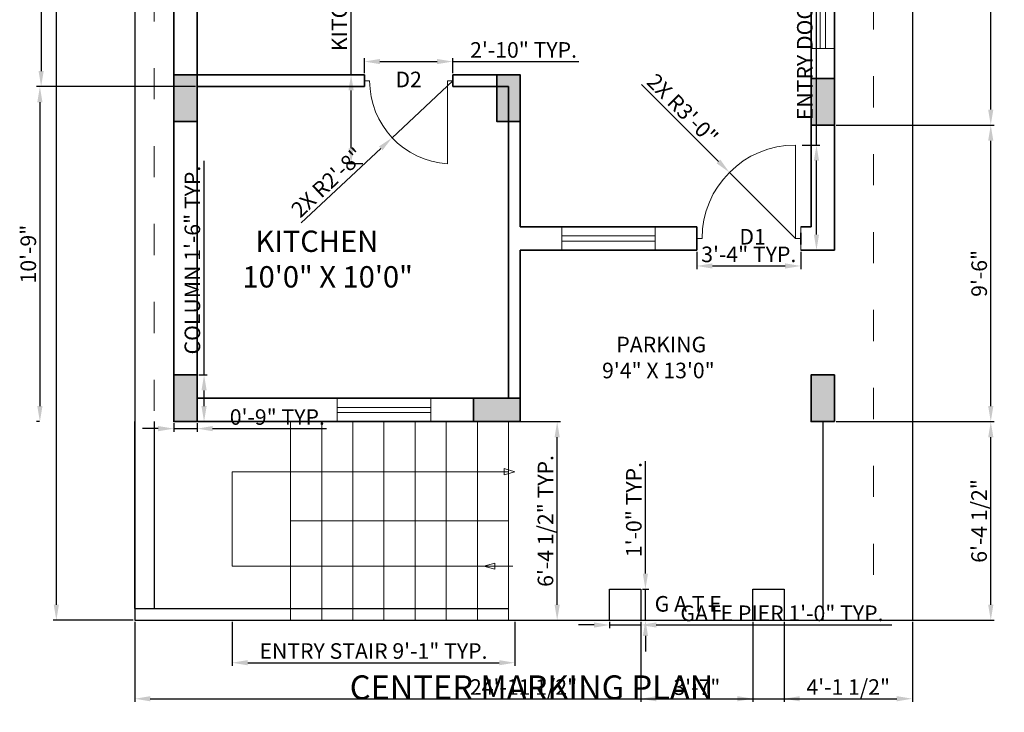
# Model space of a CAD drawing. Units: inches. Extents: x 40559 to 41508, y 131086 to 132358.
# Tile 3 of 5: x 41129 to 41508, y 131086 to 131353. Entities that reach past the tile are written whole.
import ezdxf

# ---------------------------------------------------------------- set-up
doc = ezdxf.new("R2010")
doc.units = ezdxf.units.IN
doc.linetypes.add('ACAD_ISO03W100', pattern=[30, 12, -18])
for name, color, linetype, lineweight in [('A-ANNO-DIMS', 2, 'Continuous', 18), ('A-ANNO-TEXT', 7, 'Continuous', 18), ('A-ANNO-TITL', 7, 'Continuous', 25), ('A-AREA-IDEN', 7, 'Continuous', 18), ('A-FLOR-OVHD', 240, 'ACAD_ISO03W100', 13), ('A-FLOR-STRS', 240, 'Continuous', 18), ('A-SITE-WALL', 7, 'Continuous', 30), ('A-WALL', 7, 'Continuous', 35), ('C-PROP', 7, 'Continuous', 25), ('Doors', 50, 'Continuous', 18), ('Windows', 70, 'Continuous', 18)]:
    doc.layers.add(name, color=color, linetype=linetype, lineweight=lineweight)
doc.layers.add('A-COLS', color=177, linetype='Continuous', lineweight=35, true_color=0x293189)
doc.styles.get("Standard").update_dxf_attribs({"font": 'arial.ttf'})
doc.dimstyles.new('ISO-25', dxfattribs={"dimtxt": 6, "dimasz": 6, "dimexe": 1.25, "dimexo": 0.625, "dimtad": 1, "dimdec": 0, "dimlunit": 3, "dimtxsty": 'Standard', "dimcen": 2.5, "dimclrd": 1, "dimclre": 1, "dimclrt": 2, "dimadec": 0, "dimazin": 0, "dimtfac": 1, "dimtdec": 0, "dimtmove": 0, "dimatfit": 3, "dimfxl": 1, "dimarcsym": 0})

# ---------------------------------------------------------------- blocks, each defined once
blk = doc.blocks.new('*D3')
at = {"layer": 'A-ANNO-DIMS', "color": 0, "lineweight": -2, "transparency": 16777216}
for p, q in [((41187.89, 131457.85), (41136.22, 131457.85)), ((41137.47, 131451.85), (41137.47, 131333.35)), ((41196.89, 131327.35), (41136.22, 131327.35))]:
    blk.add_line(p, q, dxfattribs=at)
at = {"layer": 'A-ANNO-DIMS', "color": 0, "transparency": 16777216}
for points in [[(41136.47, 131451.85), (41138.47, 131451.85), (41137.47, 131457.85)], [(41136.47, 131333.35), (41138.47, 131333.35), (41137.47, 131327.35)]]:
    blk.add_solid(points, dxfattribs=at)
at = {"layer": 'Defpoints', "color": 0, "transparency": 16777216}
for p in [(41188.52, 131457.85), (41137.47, 131327.35), (41197.52, 131327.35)]:
    blk.add_point(p, dxfattribs=at)
at = {"layer": 'A-ANNO-DIMS', "color": 0, "transparency": 16777216, "insert": (41133.78, 131392.6), "char_height": 6, "attachment_point": 5, "rotation": 90}
blk.add_mtext('10\'-11"', dxfattribs=at)
blk = doc.blocks.new('*D4')
at = {"layer": 'A-ANNO-DIMS', "color": 0, "lineweight": -2, "transparency": 16777216}
for p, q in [((41136.84, 131327.35), (41135.73, 131327.35)), ((41136.98, 131321.35), (41136.98, 131204.35)), ((41136.84, 131198.35), (41135.73, 131198.35))]:
    blk.add_line(p, q, dxfattribs=at)
at = {"layer": 'A-ANNO-DIMS', "color": 0, "transparency": 16777216}
for points in [[(41135.98, 131321.35), (41137.98, 131321.35), (41136.98, 131327.35)], [(41135.98, 131204.35), (41137.98, 131204.35), (41136.98, 131198.35)]]:
    blk.add_solid(points, dxfattribs=at)
at = {"layer": 'Defpoints', "color": 0, "transparency": 16777216}
for p in [(41137.47, 131327.35), (41136.98, 131198.35), (41137.47, 131198.35)]:
    blk.add_point(p, dxfattribs=at)
at = {"layer": 'A-ANNO-DIMS', "color": 0, "transparency": 16777216, "insert": (41133.29, 131262.85), "char_height": 6, "attachment_point": 5, "rotation": 90}
blk.add_mtext('10\'-9"', dxfattribs=at)
blk = doc.blocks.new('WIN-36IN')
for p, q in [((0, 5.5), (36, 5.5)), ((0, 3.5), (36, 3.5))]:
    blk.add_line(p, q)
blk.add_lwpolyline([(0, 9), (36, 9), (36, 0), (0, 0)], close=True)
blk = doc.blocks.new('WIN-38IN')
for p, q in [((0, 5.5), (38, 5.5)), ((0, 3.5), (38, 3.5))]:
    blk.add_line(p, q)
blk.add_lwpolyline([(0, 9), (38, 9), (38, 0), (0, 0)], close=True)
blk = doc.blocks.new('DOOR-KITCHEN-34IN')
for p, q in [((34, 29.75), (34, 34.25)), ((34, 29.75), (34, 34.25)), ((0, 32), (2, 32)), ((34, 32), (32, 32)), ((32, 32), (32, 0))]:
    blk.add_line(p, q)
blk.add_arc((34.07, 32), 32.07, 180, 266.3048)
blk = doc.blocks.new('DOOR-ENTRY-40IN')
for p, q in [((38, 4.5), (38, 40.5)), ((40, 9), (40, 0)), ((2, 4.5), (0, 4.5)), ((40, 4.5), (38, 4.5)), ((40, 6.75), (40, 2.25))]:
    blk.add_line(p, q)
blk.add_arc((38, 4.5), 36, 90, 180)
blk = doc.blocks.new('COL-9X18IN')
h = blk.add_hatch(color=256)
h.dxf.hatch_style = 1
h.paths.add_polyline_path([(9, 18), (0, 18), (0, 0), (9, 0)])
blk.add_lwpolyline([(0, 18), (9, 18), (9, 0), (0, 0)], close=True)
blk = doc.blocks.new('ENTRY-STAIR-PLAN')
for p, q in [((22.49, 76.5), (22.49, 0)), ((34.49, 76.5), (34.49, 0)), ((46.49, 76.5), (46.49, 0)), ((58.49, 76.5), (58.49, 0)), ((70.49, 76.5), (70.49, 0)), ((82.49, 76.5), (82.49, 0)), ((94.49, 76.5), (94.49, 0)), ((106.49, 76.5), (106.49, 0)), ((106.49, 57.22), (0, 57.22)), ((0, 57.22), (0, 20.84)), ((97.68, 57.22), (104.71, 57.22)), ((104.71, 57.22), (104.71, 58.4)), ((104.71, 58.4), (108.86, 57.22)), ((104.71, 57.22), (104.71, 56.03)), ((104.71, 56.03), (108.86, 57.22)), ((106.49, 38.25), (22.49, 38.25)), ((0, 20.84), (106.49, 20.84)), ((101.13, 22.03), (96.98, 20.84)), ((101.13, 19.65), (96.98, 20.84)), ((101.13, 20.84), (101.13, 22.03)), ((108.16, 20.84), (101.13, 20.84)), ((101.13, 20.84), (101.13, 19.65))]:
    blk.add_line(p, q)
blk = doc.blocks.new('GATE-PIER-12IN')
for p, q in [((0, 0), (0, 12)), ((0, 12), (12, 12)), ((0, 0), (0, 12)), ((0, 12), (12, 12)), ((12, 12), (12, 0)), ((12, 12), (12, 0))]:
    blk.add_line(p, q)
blk = doc.blocks.new('*D32')
at = {"layer": 'A-ANNO-DIMS', "color": 1, "lineweight": -2, "transparency": 16777216}
for p, q in [((41200.22, 131216.35), (41200.22, 131298.76)), ((41198.14, 131216.35), (41201.47, 131216.35)), ((41200.22, 131204.35), (41200.22, 131210.35)), ((41198.14, 131198.35), (41201.47, 131198.35))]:
    blk.add_line(p, q, dxfattribs=at)
at = {"layer": 'A-ANNO-DIMS', "color": 1, "transparency": 16777216}
for points in [[(41199.22, 131210.35), (41201.22, 131210.35), (41200.22, 131216.35)], [(41199.22, 131204.35), (41201.22, 131204.35), (41200.22, 131198.35)]]:
    blk.add_solid(points, dxfattribs=at)
at = {"layer": 'Defpoints', "color": 0, "transparency": 16777216}
for p in [(41197.52, 131216.35), (41200.22, 131216.35), (41197.52, 131198.35)]:
    blk.add_point(p, dxfattribs=at)
at = {"layer": 'A-ANNO-DIMS', "color": 2, "transparency": 16777216, "insert": (41196.49, 131260.55), "char_height": 6, "attachment_point": 5, "rotation": 90}
blk.add_mtext('COLUMN 1\'-6" TYP.', dxfattribs=at)
blk = doc.blocks.new('*D33')
at = {"layer": 'A-ANNO-DIMS', "color": 1, "lineweight": -2, "transparency": 16777216}
for p, q in [((41182.52, 131195.65), (41176.52, 131195.65)), ((41188.52, 131197.73), (41188.52, 131194.4)), ((41188.52, 131195.65), (41197.52, 131195.65)), ((41197.52, 131197.73), (41197.52, 131194.4)), ((41203.52, 131195.65), (41247.34, 131195.65))]:
    blk.add_line(p, q, dxfattribs=at)
at = {"layer": 'A-ANNO-DIMS', "color": 1, "transparency": 16777216}
for points in [[(41182.52, 131196.65), (41182.52, 131194.65), (41188.52, 131195.65)], [(41203.52, 131196.65), (41203.52, 131194.65), (41197.52, 131195.65)]]:
    blk.add_solid(points, dxfattribs=at)
at = {"layer": 'Defpoints', "color": 0, "transparency": 16777216}
for p in [(41188.52, 131198.35), (41197.52, 131198.35), (41197.52, 131195.65)]:
    blk.add_point(p, dxfattribs=at)
at = {"layer": 'A-ANNO-DIMS', "color": 2, "transparency": 16777216, "insert": (41228.43, 131199.34), "char_height": 6, "attachment_point": 5}
blk.add_mtext('0\'-9" TYP.', dxfattribs=at)
blk = doc.blocks.new('*D42')
at = {"layer": 'A-ANNO-DIMS', "color": 1, "lineweight": -2, "transparency": 16777216}
for p, q in [((41256.84, 131331.85), (41256.84, 131460.64)), ((41261.35, 131331.85), (41255.59, 131331.85)), ((41256.84, 131303.6), (41256.84, 131325.85)), ((41261.35, 131297.6), (41255.59, 131297.6))]:
    blk.add_line(p, q, dxfattribs=at)
at = {"layer": 'A-ANNO-DIMS', "color": 1, "transparency": 16777216}
for points in [[(41255.84, 131325.85), (41257.84, 131325.85), (41256.84, 131331.85)], [(41255.84, 131303.6), (41257.84, 131303.6), (41256.84, 131297.6)]]:
    blk.add_solid(points, dxfattribs=at)
at = {"layer": 'Defpoints', "color": 0, "transparency": 16777216}
for p in [(41256.84, 131331.85), (41261.98, 131331.85), (41261.98, 131297.6)]:
    blk.add_point(p, dxfattribs=at)
at = {"layer": 'A-ANNO-DIMS', "color": 2, "transparency": 16777216, "insert": (41253.11, 131399.25), "char_height": 6, "attachment_point": 5, "rotation": 90}
blk.add_mtext('KITCHEN DOOR 2\'-10 1/2" TYP.', dxfattribs=at)
blk = doc.blocks.new('*D43')
at = {"layer": 'A-ANNO-DIMS', "color": 1, "lineweight": -2, "transparency": 16777216}
for p, q in [((41261.98, 131332.48), (41261.98, 131338.24)), ((41267.98, 131336.99), (41289.98, 131336.99)), ((41295.98, 131332.48), (41295.98, 131338.24)), ((41295.98, 131336.99), (41344.56, 131336.99))]:
    blk.add_line(p, q, dxfattribs=at)
at = {"layer": 'A-ANNO-DIMS', "color": 1, "transparency": 16777216}
for points in [[(41267.98, 131337.99), (41267.98, 131335.99), (41261.98, 131336.99)], [(41289.98, 131337.99), (41289.98, 131335.99), (41295.98, 131336.99)]]:
    blk.add_solid(points, dxfattribs=at)
at = {"layer": 'Defpoints', "color": 0, "transparency": 16777216}
for p in [(41295.98, 131336.99), (41261.98, 131331.85), (41295.98, 131331.85)]:
    blk.add_point(p, dxfattribs=at)
at = {"layer": 'A-ANNO-DIMS', "color": 2, "transparency": 16777216, "insert": (41323.27, 131340.68), "char_height": 6, "attachment_point": 5}
blk.add_mtext('2\'-10" TYP.', dxfattribs=at)
blk = doc.blocks.new('*D44')
at = {"layer": 'A-ANNO-DIMS', "color": 1, "lineweight": -2, "transparency": 16777216}
for p, q in [((41436.09, 131304.85), (41436.09, 131420.55)), ((41430.64, 131304.85), (41437.34, 131304.85)), ((41436.09, 131270.35), (41436.09, 131298.85)), ((41430.64, 131264.35), (41437.34, 131264.35))]:
    blk.add_line(p, q, dxfattribs=at)
at = {"layer": 'A-ANNO-DIMS', "color": 1, "transparency": 16777216}
for points in [[(41435.09, 131298.85), (41437.09, 131298.85), (41436.09, 131304.85)], [(41435.09, 131270.35), (41437.09, 131270.35), (41436.09, 131264.35)]]:
    blk.add_solid(points, dxfattribs=at)
at = {"layer": 'Defpoints', "color": 0, "transparency": 16777216}
for p in [(41430.02, 131304.85), (41436.09, 131304.85), (41430.02, 131264.35)]:
    blk.add_point(p, dxfattribs=at)
at = {"layer": 'A-ANNO-DIMS', "color": 2, "transparency": 16777216, "insert": (41432.36, 131365.7), "char_height": 6, "attachment_point": 5, "rotation": 90}
blk.add_mtext('ENTRY DOOR 3\'-4 1/2" TYP.', dxfattribs=at)
blk = doc.blocks.new('*D45')
at = {"layer": 'A-ANNO-DIMS', "color": 1, "lineweight": -2, "transparency": 16777216}
for p, q in [((41390.02, 131263.73), (41390.02, 131257.03)), ((41430.02, 131263.73), (41430.02, 131257.03)), ((41396.02, 131258.28), (41424.02, 131258.28))]:
    blk.add_line(p, q, dxfattribs=at)
at = {"layer": 'A-ANNO-DIMS', "color": 1, "transparency": 16777216}
for points in [[(41396.02, 131259.28), (41396.02, 131257.28), (41390.02, 131258.28)], [(41424.02, 131259.28), (41424.02, 131257.28), (41430.02, 131258.28)]]:
    blk.add_solid(points, dxfattribs=at)
at = {"layer": 'Defpoints', "color": 0, "transparency": 16777216}
for p in [(41390.02, 131264.35), (41430.02, 131264.35), (41430.02, 131258.28)]:
    blk.add_point(p, dxfattribs=at)
at = {"layer": 'A-ANNO-DIMS', "color": 2, "transparency": 16777216, "insert": (41410.02, 131261.97), "char_height": 6, "attachment_point": 5}
blk.add_mtext('3\'-4" TYP.', dxfattribs=at)
blk = doc.blocks.new('*D50')
at = {"layer": 'A-ANNO-DIMS', "color": 1, "lineweight": -2, "transparency": 16777216}
for p, q in [((41350.41, 131120.05), (41344.41, 131120.05)), ((41356.41, 131121.23), (41356.41, 131118.8)), ((41356.41, 131120.05), (41368.41, 131120.05)), ((41368.41, 131121.23), (41368.41, 131118.8)), ((41374.41, 131120.05), (41465.18, 131120.05))]:
    blk.add_line(p, q, dxfattribs=at)
at = {"layer": 'A-ANNO-DIMS', "color": 1, "transparency": 16777216}
for points in [[(41350.41, 131121.05), (41350.41, 131119.05), (41356.41, 131120.05)], [(41374.41, 131121.05), (41374.41, 131119.05), (41368.41, 131120.05)]]:
    blk.add_solid(points, dxfattribs=at)
at = {"layer": 'Defpoints', "color": 0, "transparency": 16777216}
for p in [(41356.41, 131121.85), (41368.41, 131121.85), (41368.41, 131120.05)]:
    blk.add_point(p, dxfattribs=at)
at = {"layer": 'A-ANNO-DIMS', "color": 2, "transparency": 16777216, "insert": (41422.79, 131123.78), "char_height": 6, "attachment_point": 5}
blk.add_mtext('GATE PIER 1\'-0" TYP.', dxfattribs=at)
blk = doc.blocks.new('*D51')
at = {"layer": 'A-ANNO-DIMS', "color": 1, "lineweight": -2, "transparency": 16777216}
for p, q in [((41370.21, 131139.85), (41370.21, 131183.11)), ((41369.04, 131133.85), (41371.46, 131133.85)), ((41370.21, 131121.85), (41370.21, 131133.85)), ((41369.04, 131121.85), (41371.46, 131121.85)), ((41370.21, 131115.85), (41370.21, 131109.85))]:
    blk.add_line(p, q, dxfattribs=at)
at = {"layer": 'A-ANNO-DIMS', "color": 1, "transparency": 16777216}
for points in [[(41369.21, 131139.85), (41371.21, 131139.85), (41370.21, 131133.85)], [(41369.21, 131115.85), (41371.21, 131115.85), (41370.21, 131121.85)]]:
    blk.add_solid(points, dxfattribs=at)
at = {"layer": 'Defpoints', "color": 0, "transparency": 16777216}
for p in [(41368.41, 131133.85), (41370.21, 131133.85), (41368.41, 131121.85)]:
    blk.add_point(p, dxfattribs=at)
at = {"layer": 'A-ANNO-DIMS', "color": 2, "transparency": 16777216, "insert": (41366.52, 131164.48), "char_height": 6, "attachment_point": 5, "rotation": 90}
blk.add_mtext('1\'-0" TYP.', dxfattribs=at)
blk = doc.blocks.new('*D60')
at = {"layer": 'A-ANNO-DIMS', "color": 1, "lineweight": -2, "transparency": 16777216}
for p, q in [((41211.03, 131121.23), (41211.03, 131104.27)), ((41319.88, 131121.23), (41319.88, 131104.27)), ((41217.03, 131105.52), (41313.88, 131105.52))]:
    blk.add_line(p, q, dxfattribs=at)
at = {"layer": 'A-ANNO-DIMS', "color": 1, "transparency": 16777216}
for points in [[(41217.03, 131106.52), (41217.03, 131104.52), (41211.03, 131105.52)], [(41313.88, 131106.52), (41313.88, 131104.52), (41319.88, 131105.52)]]:
    blk.add_solid(points, dxfattribs=at)
at = {"layer": 'Defpoints', "color": 0, "transparency": 16777216}
for p in [(41211.03, 131121.85), (41319.88, 131121.85), (41319.88, 131105.52)]:
    blk.add_point(p, dxfattribs=at)
at = {"layer": 'A-ANNO-DIMS', "color": 2, "transparency": 16777216, "insert": (41265.46, 131109.25), "char_height": 6, "attachment_point": 5}
blk.add_mtext('ENTRY STAIR 9\'-1" TYP.', dxfattribs=at)
blk = doc.blocks.new('*D61')
at = {"layer": 'A-ANNO-DIMS', "color": 1, "lineweight": -2, "transparency": 16777216}
for p, q in [((41320.51, 131198.35), (41337.46, 131198.35)), ((41336.21, 131127.85), (41336.21, 131192.35)), ((41320.51, 131121.85), (41337.46, 131121.85))]:
    blk.add_line(p, q, dxfattribs=at)
at = {"layer": 'A-ANNO-DIMS', "color": 1, "transparency": 16777216}
for points in [[(41335.21, 131192.35), (41337.21, 131192.35), (41336.21, 131198.35)], [(41335.21, 131127.85), (41337.21, 131127.85), (41336.21, 131121.85)]]:
    blk.add_solid(points, dxfattribs=at)
at = {"layer": 'Defpoints', "color": 0, "transparency": 16777216}
for p in [(41319.88, 131198.35), (41336.21, 131198.35), (41319.88, 131121.85)]:
    blk.add_point(p, dxfattribs=at)
at = {"layer": 'A-ANNO-DIMS', "color": 2, "transparency": 16777216, "insert": (41332.49, 131160.1), "char_height": 6, "attachment_point": 5, "rotation": 90}
blk.add_mtext('6\'-4 1/2" TYP.', dxfattribs=at)
blk = doc.blocks.new('*D71')
at = {"layer": 'A-ANNO-DIMS', "color": 1, "lineweight": -2, "transparency": 16777216}
for p, q in [((41173.52, 131121.23), (41173.52, 131090.4)), ((41473.02, 131121.23), (41473.02, 131090.4)), ((41179.52, 131091.65), (41467.02, 131091.65))]:
    blk.add_line(p, q, dxfattribs=at)
at = {"layer": 'A-ANNO-DIMS', "color": 1, "transparency": 16777216}
for points in [[(41179.52, 131092.65), (41179.52, 131090.65), (41173.52, 131091.65)], [(41467.02, 131092.65), (41467.02, 131090.65), (41473.02, 131091.65)]]:
    blk.add_solid(points, dxfattribs=at)
at = {"layer": 'Defpoints', "color": 0, "transparency": 16777216}
for p in [(41173.52, 131121.85), (41473.02, 131121.85), (41473.02, 131091.65)]:
    blk.add_point(p, dxfattribs=at)
at = {"layer": 'A-ANNO-DIMS', "color": 2, "transparency": 16777216, "insert": (41323.27, 131095.38), "char_height": 6, "attachment_point": 5}
blk.add_mtext('24\'-11 1/2"', dxfattribs=at)
blk = doc.blocks.new('*D72')
at = {"layer": 'A-ANNO-DIMS', "color": 1, "lineweight": -2, "transparency": 16777216}
for p, q in [((41172.89, 131667.35), (41142.07, 131667.35)), ((41143.32, 131127.85), (41143.32, 131661.35)), ((41172.89, 131121.85), (41142.07, 131121.85))]:
    blk.add_line(p, q, dxfattribs=at)
at = {"layer": 'A-ANNO-DIMS', "color": 1, "transparency": 16777216}
for points in [[(41142.32, 131661.35), (41144.32, 131661.35), (41143.32, 131667.35)], [(41142.32, 131127.85), (41144.32, 131127.85), (41143.32, 131121.85)]]:
    blk.add_solid(points, dxfattribs=at)
at = {"layer": 'Defpoints', "color": 0, "transparency": 16777216}
for p in [(41143.32, 131667.35), (41173.52, 131667.35), (41173.52, 131121.85)]:
    blk.add_point(p, dxfattribs=at)
at = {"layer": 'A-ANNO-DIMS', "color": 2, "transparency": 16777216, "insert": (41139.59, 131394.6), "char_height": 6, "attachment_point": 5, "rotation": 90}
blk.add_mtext('45\'-5 1/2"', dxfattribs=at)
blk = doc.blocks.new('*D75')
at = {"layer": 'A-ANNO-DIMS', "color": 1, "lineweight": -2, "transparency": 16777216}
for p, q in [((41443.64, 131198.35), (41504.47, 131198.35)), ((41503.22, 131127.85), (41503.22, 131192.35)), ((41439.14, 131121.85), (41504.47, 131121.85))]:
    blk.add_line(p, q, dxfattribs=at)
at = {"layer": 'A-ANNO-DIMS', "color": 1, "transparency": 16777216}
for points in [[(41502.22, 131192.35), (41504.22, 131192.35), (41503.22, 131198.35)], [(41502.22, 131127.85), (41504.22, 131127.85), (41503.22, 131121.85)]]:
    blk.add_solid(points, dxfattribs=at)
at = {"layer": 'Defpoints', "color": 0, "transparency": 16777216}
for p in [(41443.02, 131198.35), (41503.22, 131198.35), (41438.52, 131121.85)]:
    blk.add_point(p, dxfattribs=at)
at = {"layer": 'A-ANNO-DIMS', "color": 2, "transparency": 16777216, "insert": (41499.49, 131160.1), "char_height": 6, "attachment_point": 5, "rotation": 90}
blk.add_mtext('6\'-4 1/2"', dxfattribs=at)
blk = doc.blocks.new('*D76')
at = {"layer": 'A-ANNO-DIMS', "color": 1, "lineweight": -2, "transparency": 16777216}
for p, q in [((41443.64, 131312.51), (41504.47, 131312.51)), ((41503.22, 131204.35), (41503.22, 131306.51)), ((41443.64, 131198.35), (41504.47, 131198.35))]:
    blk.add_line(p, q, dxfattribs=at)
at = {"layer": 'A-ANNO-DIMS', "color": 1, "transparency": 16777216}
for points in [[(41502.22, 131306.51), (41504.22, 131306.51), (41503.22, 131312.51)], [(41502.22, 131204.35), (41504.22, 131204.35), (41503.22, 131198.35)]]:
    blk.add_solid(points, dxfattribs=at)
at = {"layer": 'Defpoints', "color": 0, "transparency": 16777216}
for p in [(41443.02, 131312.51), (41503.22, 131312.51), (41443.02, 131198.35)]:
    blk.add_point(p, dxfattribs=at)
at = {"layer": 'A-ANNO-DIMS', "color": 2, "transparency": 16777216, "insert": (41499.53, 131255.43), "char_height": 6, "attachment_point": 5, "rotation": 90}
blk.add_mtext('9\'-6"', dxfattribs=at)
blk = doc.blocks.new('*D77')
at = {"layer": 'A-ANNO-DIMS', "color": 1, "lineweight": -2, "transparency": 16777216}
for p, q in [((41443.64, 131441.85), (41504.47, 131441.85)), ((41503.22, 131318.51), (41503.22, 131435.85)), ((41443.64, 131312.51), (41504.47, 131312.51))]:
    blk.add_line(p, q, dxfattribs=at)
at = {"layer": 'A-ANNO-DIMS', "color": 1, "transparency": 16777216}
for points in [[(41502.22, 131435.85), (41504.22, 131435.85), (41503.22, 131441.85)], [(41502.22, 131318.51), (41504.22, 131318.51), (41503.22, 131312.51)]]:
    blk.add_solid(points, dxfattribs=at)
at = {"layer": 'Defpoints', "color": 0, "transparency": 16777216}
for p in [(41443.02, 131441.85), (41503.22, 131441.85), (41443.02, 131312.51)]:
    blk.add_point(p, dxfattribs=at)
at = {"layer": 'A-ANNO-DIMS', "color": 2, "transparency": 16777216, "insert": (41499.49, 131377.18), "char_height": 6, "attachment_point": 5, "rotation": 90}
blk.add_mtext('10\'-9 1/2"', dxfattribs=at)
blk = doc.blocks.new('*D80')
at = {"layer": 'A-ANNO-DIMS', "color": 1, "lineweight": -2, "transparency": 16777216}
for p, q in [((41368.41, 131121.23), (41368.41, 131090.4)), ((41411.64, 131121.23), (41411.64, 131090.4)), ((41374.41, 131091.65), (41405.64, 131091.65))]:
    blk.add_line(p, q, dxfattribs=at)
at = {"layer": 'A-ANNO-DIMS', "color": 1, "transparency": 16777216}
for points in [[(41374.41, 131092.65), (41374.41, 131090.65), (41368.41, 131091.65)], [(41405.64, 131092.65), (41405.64, 131090.65), (41411.64, 131091.65)]]:
    blk.add_solid(points, dxfattribs=at)
at = {"layer": 'Defpoints', "color": 0, "transparency": 16777216}
for p in [(41368.41, 131121.85), (41411.64, 131121.85), (41411.64, 131091.65)]:
    blk.add_point(p, dxfattribs=at)
at = {"layer": 'A-ANNO-DIMS', "color": 2, "transparency": 16777216, "insert": (41390.03, 131095.34), "char_height": 6, "attachment_point": 5}
blk.add_mtext('3\'-7"', dxfattribs=at)
blk = doc.blocks.new('*D81')
at = {"layer": 'A-ANNO-DIMS', "color": 1, "lineweight": -2, "transparency": 16777216}
for p, q in [((41423.64, 131121.23), (41423.64, 131090.4)), ((41473.02, 131121.23), (41473.02, 131090.4)), ((41429.64, 131091.65), (41467.02, 131091.65))]:
    blk.add_line(p, q, dxfattribs=at)
at = {"layer": 'A-ANNO-DIMS', "color": 1, "transparency": 16777216}
for points in [[(41429.64, 131092.65), (41429.64, 131090.65), (41423.64, 131091.65)], [(41467.02, 131092.65), (41467.02, 131090.65), (41473.02, 131091.65)]]:
    blk.add_solid(points, dxfattribs=at)
at = {"layer": 'Defpoints', "color": 0, "transparency": 16777216}
for p in [(41423.64, 131121.85), (41473.02, 131121.85), (41473.02, 131091.65)]:
    blk.add_point(p, dxfattribs=at)
at = {"layer": 'A-ANNO-DIMS', "color": 2, "transparency": 16777216, "insert": (41448.33, 131095.38), "char_height": 6, "attachment_point": 5}
blk.add_mtext('4\'-1 1/2"', dxfattribs=at)
blk = doc.blocks.new('*D103')
at = {"layer": 'A-ANNO-DIMS', "color": 1, "lineweight": -2, "transparency": 16777216}
for p, q in [((41368.66, 131328.2), (41398.32, 131298.55)), ((41428.02, 131268.85), (41402.56, 131294.31))]:
    blk.add_line(p, q, dxfattribs=at)
at = {"layer": 'A-ANNO-DIMS', "color": 1, "transparency": 16777216}
blk.add_solid([(41399.03, 131299.26), (41397.61, 131297.84), (41402.56, 131294.31)], dxfattribs=at)
at = {"layer": 'Defpoints', "color": 0, "transparency": 16777216}
for p in [(41402.56, 131294.31), (41428.02, 131268.85)]:
    blk.add_point(p, dxfattribs=at)
at = {"layer": 'A-ANNO-DIMS', "color": 2, "transparency": 16777216, "insert": (41383.98, 131318.11), "char_height": 6, "attachment_point": 5, "rotation": 315.0003}
blk.add_mtext('2X R3\'-0"', dxfattribs=at)
blk = doc.blocks.new('*D104')
at = {"layer": 'A-ANNO-DIMS', "color": 1, "lineweight": -2, "transparency": 16777216}
for p, q in [((41296.04, 131329.6), (41272.65, 131307.67)), ((41237.68, 131274.88), (41268.27, 131303.57))]:
    blk.add_line(p, q, dxfattribs=at)
at = {"layer": 'A-ANNO-DIMS', "color": 1, "transparency": 16777216}
blk.add_solid([(41267.59, 131304.29), (41268.96, 131302.84), (41272.65, 131307.67)], dxfattribs=at)
at = {"layer": 'Defpoints', "color": 0, "transparency": 16777216}
for p in [(41296.04, 131329.6), (41272.65, 131307.67)]:
    blk.add_point(p, dxfattribs=at)
at = {"layer": 'A-ANNO-DIMS', "color": 2, "transparency": 16777216, "insert": (41248.26, 131289.86), "char_height": 6, "attachment_point": 5, "rotation": 43.1521}
blk.add_mtext('2X R2\'-8"', dxfattribs=at)

msp = doc.modelspace()

# ---------------------------------------------------------------- linework, layer by layer
at = {"layer": 'A-FLOR-OVHD'}
for p, q in [((41181.02, 131202.46), (41181.02, 131661.35)), ((41458.02, 131661.35), (41458.02, 131121.85))]:
    msp.add_line(p, q, dxfattribs=at)
at = {"layer": 'A-SITE-WALL'}
for p, q in [((41173.52, 131126.35), (41173.52, 131198.35)), ((41181.02, 131198.35), (41181.02, 131126.35)), ((41438.52, 131198.35), (41438.52, 131121.85)), ((41173.52, 131126.35), (41317.52, 131126.35)), ((41173.52, 131121.85), (41317.52, 131121.85))]:
    msp.add_line(p, q, dxfattribs=at)
at = {"layer": 'A-WALL'}
for p, q in [((41188.52, 131655.35), (41188.52, 131198.35)), ((41443.02, 131655.35), (41443.02, 131264.35)), ((41197.52, 131646.35), (41197.52, 131207.35)), ((41434.02, 131646.35), (41434.02, 131273.35)), ((41197.52, 131331.85), (41261.98, 131331.85)), ((41261.98, 131327.35), (41261.98, 131331.85)), ((41295.98, 131327.35), (41295.98, 131331.85)), ((41295.98, 131331.85), (41322.02, 131331.85)), ((41322.02, 131331.85), (41322.02, 131273.35)), ((41197.52, 131327.35), (41261.98, 131327.35)), ((41197.52, 131327.35), (41197.52, 131207.35)), ((41295.98, 131327.35), (41317.52, 131327.35)), ((41317.52, 131327.35), (41317.52, 131207.35)), ((41322.02, 131273.35), (41390.02, 131273.35)), ((41390.02, 131273.35), (41390.02, 131264.35)), ((41430.02, 131273.35), (41434.02, 131273.35)), ((41430.02, 131271.1), (41430.02, 131266.6)), ((41322.02, 131264.35), (41390.02, 131264.35)), ((41322.02, 131264.35), (41322.02, 131198.35)), ((41430.02, 131264.35), (41443.02, 131264.35)), ((41197.52, 131207.35), (41317.52, 131207.35)), ((41188.52, 131198.35), (41322.02, 131198.35))]:
    msp.add_line(p, q, dxfattribs=at)
at = {"layer": 'C-PROP'}
for p, q in [((41173.52, 131667.35), (41173.52, 131121.85)), ((41473.02, 131667.35), (41473.02, 131121.85)), ((41173.52, 131121.85), (41473.02, 131121.85))]:
    msp.add_line(p, q, dxfattribs=at)

# ---------------------------------------------------------------- block references
at = {"layer": 'A-COLS'}
for p in [(41188.52, 131313.85), (41188.52, 131198.35)]:
    msp.add_blockref('COL-9X18IN', p, dxfattribs=at)
for p, rotation in [((41322.02, 131331.85), 180), ((41443.02, 131330.51), 180), ((41443.02, 131216.35), 180), ((41304.02, 131207.35), 270.0000000000411)]:
    msp.add_blockref('COL-9X18IN', p, dxfattribs=dict(at, rotation=rotation))
at = {"layer": 'A-FLOR-STRS'}
msp.add_blockref('ENTRY-STAIR-PLAN', (41211.03, 131121.85), dxfattribs=at)
at = {"layer": 'A-SITE-WALL'}
for p in [(41356.41, 131121.85), (41411.64, 131121.85)]:
    msp.add_blockref('GATE-PIER-12IN', p, dxfattribs=at)
at = {"layer": 'Doors'}
for name, p in [('DOOR-KITCHEN-34IN', (41261.98, 131297.6)), ('DOOR-ENTRY-40IN', (41390.02, 131264.35))]:
    msp.add_blockref(name, p, dxfattribs=at)
at = {"layer": 'Windows', "rotation": 269.9999999999867}
msp.add_blockref('WIN-38IN', (41434.02, 131380.06), dxfattribs=at)
at = {"layer": 'Windows'}
for p in [(41338.02, 131264.35), (41251.52, 131198.35)]:
    msp.add_blockref('WIN-36IN', p, dxfattribs=at)

# ---------------------------------------------------------------- texts
at = {"layer": 'A-ANNO-TEXT', "char_height": 6, "attachment_point": 1}
for s, width, insert in [('{D2}', 6, (41273.93, 131333.08)), ('{D1}', 6, (41406.4, 131272.54)), ('{\\fArial|b1|i0|c0|p34;G A T E}', 37.8561, (41373.79, 131131.19))]:
    msp.add_mtext_dynamic_manual_height_columns(s, width=width, gutter_width=12.5, heights=[0], dxfattribs=dict(at, insert=insert))
at = {"layer": 'A-ANNO-TITL', "insert": (41256.32, 131100.64), "char_height": 9.2211, "attachment_point": 1}
msp.add_mtext_dynamic_manual_height_columns('{\\fArial|b1|i0|c0|p34;CENTER MARKING PLAN}', width=193.072, gutter_width=19.21, heights=[0], dxfattribs=at)
at = {"layer": 'A-AREA-IDEN', "attachment_point": 1}
for s, width, gutter_width, insert, char_height in [('{\\fArial|b1|i0|c0|p34;  KITCHEN\\P10\'0" X 10\'0"}', 121.5689, 17.12, (41215, 131271.91), 8.2185), ('{\\fArial|b1|i0|c0|p34;   PARKING\\P9\'4" X 13\'0"}', 54.4487, 12.5, (41353.51, 131231.04), 6)]:
    msp.add_mtext_dynamic_manual_height_columns(s, width=width, gutter_width=gutter_width, heights=[0], dxfattribs=dict(at, insert=insert, char_height=char_height))

# ---------------------------------------------------------------- dimensions: what is measured, and where the dimension line sits
at = {"layer": 'A-ANNO-DIMS'}
for base, p1, p2, override, picture, middle in [((41143.32, 131667.35), (41173.52, 131121.85), (41173.52, 131667.35), {"dimdec": 1, "dimlfac": 1, "dimrnd": 0, "dimzin": 1, "dimdsep": 46, "dimlunit": 4, "dimfrac": 2}, '*D72', (41139.59, 131394.6)), ((41137.46517777, 131327.35041044), (41188.51685623, 131457.85041044), (41197.51685623, 131327.35041044), {"dimclrd": 0, "dimclre": 0, "dimclrt": 0}, '*D3', (41133.77673984, 131392.60041044)), ((41503.22, 131441.85), (41443.02, 131312.51), (41443.02, 131441.85), {"dimdec": 1, "dimlfac": 1, "dimrnd": 0, "dimzin": 1, "dimdsep": 46, "dimlunit": 4, "dimfrac": 2}, '*D77', (41499.49, 131377.18)), ((41136.98, 131198.35), (41137.47, 131327.35), (41137.47, 131198.35), {"dimclrd": 0, "dimclre": 0, "dimclrt": 0}, '*D4', (41133.29, 131262.85)), ((41503.22, 131312.51), (41443.02, 131198.35), (41443.02, 131312.51), {"dimdec": 1, "dimlfac": 1, "dimrnd": 0, "dimzin": 1, "dimdsep": 46, "dimlunit": 4, "dimfrac": 2}, '*D76', (41499.53, 131255.43)), ((41503.22, 131198.35), (41438.52, 131121.85), (41443.02, 131198.35), {"dimdec": 1, "dimlfac": 1, "dimrnd": 0, "dimzin": 1, "dimdsep": 46, "dimlunit": 4, "dimfrac": 2}, '*D75', (41499.49, 131160.1))]:
    dim = msp.add_linear_dim(base=base, p1=p1, p2=p2, angle=90, dimstyle='ISO-25', override=override, dxfattribs=at)
    dim.commit()
    dim.dimension.update_dxf_attribs({"geometry": picture, "text_midpoint": middle})
for base, p1, p2, text, picture, middle in [((41256.83955995, 131331.85041044), (41261.97705995, 131297.60041044), (41261.97705995, 131331.85041044), 'KITCHEN DOOR <> TYP.', '*D42', (41253.11019433, 131399.24689748)), ((41436.09, 131304.85), (41430.02, 131264.35), (41430.02, 131304.85), 'ENTRY DOOR <> TYP.', '*D44', (41432.36, 131365.7)), ((41200.22, 131216.35), (41197.52, 131198.35), (41197.52, 131216.35), 'COLUMN <> TYP.', '*D32', (41196.49, 131260.55)), ((41336.21, 131198.35), (41319.88, 131121.85), (41319.88, 131198.35), '<> TYP.', '*D61', (41332.49, 131160.1)), ((41370.21, 131133.85), (41368.41, 131121.85), (41368.41, 131133.85), '<> TYP.', '*D51', (41366.52, 131164.48))]:
    dim = msp.add_linear_dim(base=base, p1=p1, p2=p2, angle=90, text=text, dimstyle='ISO-25', override={"dimdec": 1, "dimlfac": 1, "dimrnd": 0, "dimzin": 1, "dimdsep": 46, "dimlunit": 4, "dimfrac": 2}, dxfattribs=at)
    dim.commit()
    dim.dimension.update_dxf_attribs({"geometry": picture, "text_midpoint": middle})
for base, p1, p2, text, picture, middle in [((41295.98, 131336.99), (41261.98, 131331.85), (41295.98, 131331.85), '<> TYP.', '*D43', (41323.27, 131340.68)), ((41430.02, 131258.28), (41390.02, 131264.35), (41430.02, 131264.35), '<> TYP.', '*D45', (41410.02, 131261.97)), ((41197.52, 131195.65), (41188.52, 131198.35), (41197.52, 131198.35), '<> TYP.', '*D33', (41228.43, 131199.34)), ((41368.41, 131120.05), (41356.41, 131121.85), (41368.41, 131121.85), 'GATE PIER <> TYP.', '*D50', (41422.79, 131123.78)), ((41319.8841, 131105.522), (41211.0283, 131121.8504), (41319.8841, 131121.8504), 'ENTRY STAIR <> TYP.', '*D60', (41265.4562, 131109.2494))]:
    dim = msp.add_linear_dim(base=base, p1=p1, p2=p2, text=text, dimstyle='ISO-25', override={"dimdec": 1, "dimlfac": 1, "dimrnd": 0, "dimzin": 1, "dimdsep": 46, "dimlunit": 4, "dimfrac": 2}, dxfattribs=at)
    dim.commit()
    dim.dimension.update_dxf_attribs({"geometry": picture, "text_midpoint": middle})
for center, mpoint, picture, middle in [((41428.02, 131268.85), (41402.56, 131294.31), '*D103', (41383.98, 131318.11)), ((41296.04, 131329.6), (41272.65, 131307.67), '*D104', (41248.26, 131289.86))]:
    dim = msp.add_radius_dim(center=center, mpoint=mpoint, text='2X <>', dimstyle='ISO-25', override={"dimdec": 1, "dimlfac": 1, "dimrnd": 0, "dimzin": 1, "dimdsep": 46, "dimlunit": 4, "dimfrac": 2}, dxfattribs=at)
    dim.commit()
    dim.dimension.update_dxf_attribs({"geometry": picture, "text_midpoint": middle})
for base, p1, p2, picture, middle in [((41473.02, 131091.65), (41173.52, 131121.85), (41473.02, 131121.85), '*D71', (41323.27, 131095.38)), ((41411.64, 131091.65), (41368.41, 131121.85), (41411.64, 131121.85), '*D80', (41390.03, 131095.34)), ((41473.02, 131091.65), (41423.64, 131121.85), (41473.02, 131121.85), '*D81', (41448.33, 131095.38))]:
    dim = msp.add_linear_dim(base=base, p1=p1, p2=p2, dimstyle='ISO-25', override={"dimdec": 1, "dimlfac": 1, "dimrnd": 0, "dimzin": 1, "dimdsep": 46, "dimlunit": 4, "dimfrac": 2}, dxfattribs=at)
    dim.commit()
    dim.dimension.update_dxf_attribs({"geometry": picture, "text_midpoint": middle})

doc.saveas('drawing.dxf')
